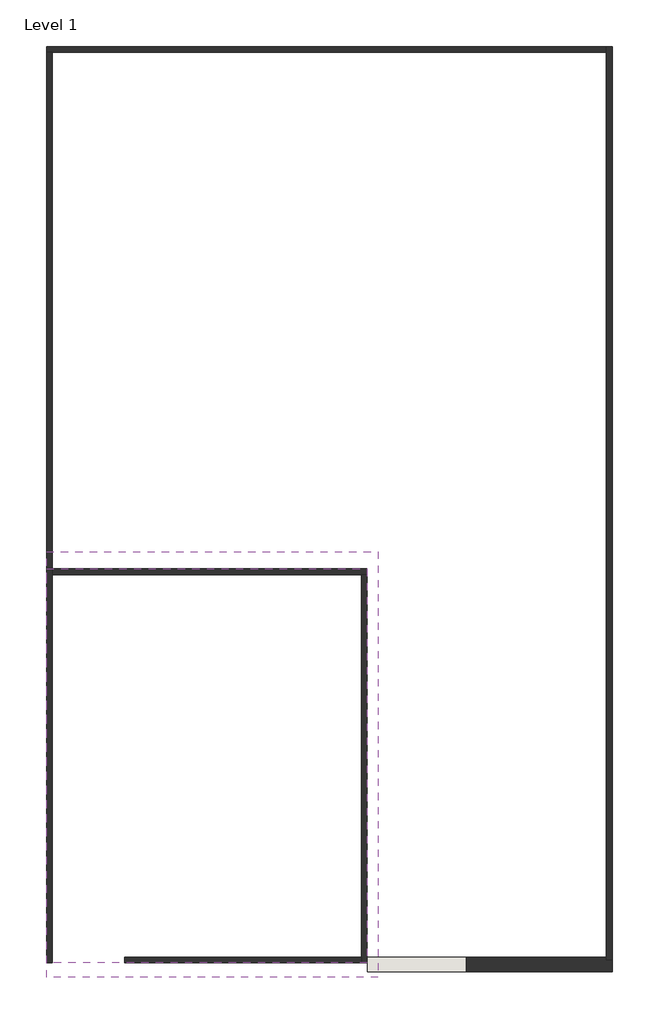
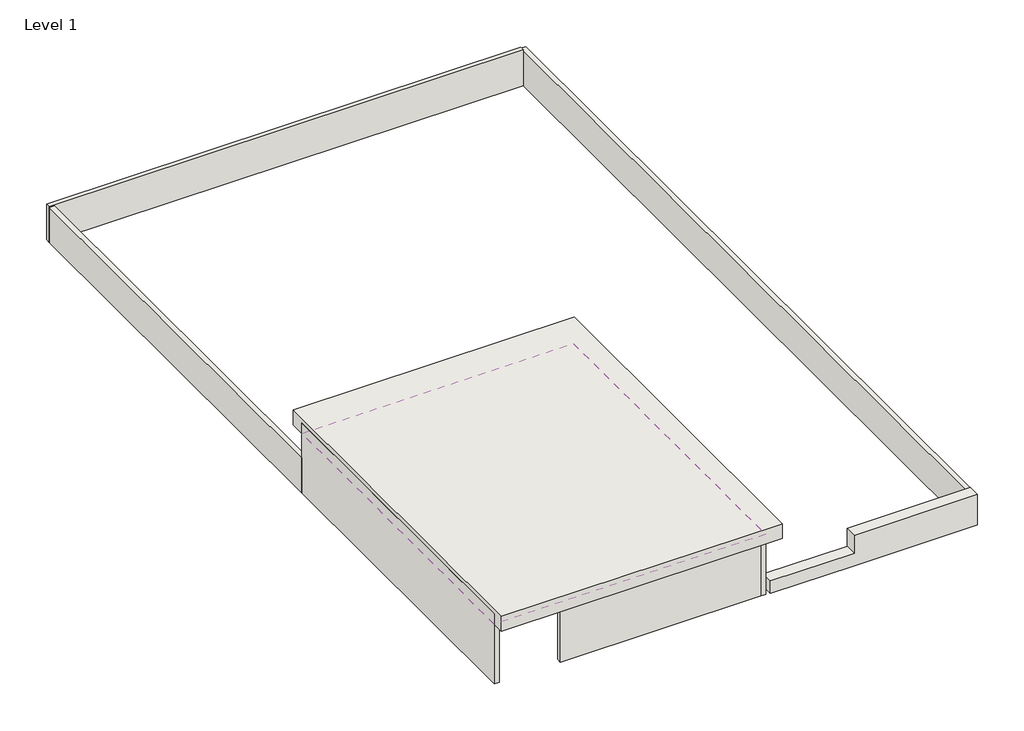
# One storey: 9 walls, 1 covering.
"""IFC4 building model written with IfcOpenShell, lengths in millimetres."""

from ifc_helpers import new_model, si_unit, frame, origin, place, context, project, spatial, polyline, outline, extrude, faceted_brep, transform, mapped, element, save
from components import walls_1_walls_1_3090deb3, walls_8_walls_8_6bca06a2

model = new_model("IFC4")

# Units and contexts
model_context = context("Model", 3, world=origin())
ifc_project = project(units=[si_unit("LENGTHUNIT", "METRE", prefix="MILLI")], contexts=[model_context])

# Site, building, storey
site = spatial("IfcSite", under=ifc_project)
building = spatial("IfcBuilding", under=site)
storey = spatial("IfcBuildingStorey", under=building, Name="Level 1", Elevation=3048.0)

# Covering
placement = place(None, origin())
element("IfcCovering", 1, ObjectType="600 x 1200mm grid", at=placement, inside=storey, context=model_context, shape_type="SweptSolid", body=[
    extrude(outline(polyline([(-7329.4383357, -6419.7210337), (-7329.4383357, -20130.9210337), (-18502.2383357, -20130.9210337), (-18502.2383357, -6419.7210337), (-7329.4383357, -6419.7210337)])), frame((0.0, 0.0, 5648.0), z_axis=(0.0, 0.0, 1.0), x_axis=(1.0, 0.0, 0.0)), (0.0, 0.0, 1.0), 52.0),
])

# Walls
element("IfcWall", 2, ObjectType="Generic - 9\"", at=placement, inside=storey, context=model_context, shape_type="SweptSolid", body=[
    extrude(outline(polyline([(-7529.4383357, -20130.9210337), (-15779.6883357, -20130.9210337), (-15779.6883357, -19930.9210337), (-7529.4383357, -19930.9210337), (-7529.4383357, -20130.9210337)])), frame((0.0, 0.0, 3048.0), z_axis=(0.0, 0.0, 1.0), x_axis=(1.0, 0.0, 0.0)), (0.0, 0.0, 1.0), 3048.0),
])
element("IfcWall", 3, ObjectType="Generic - 9\"", at=placement, inside=storey, context=model_context, shape_type="Brep", body=[
    faceted_brep([(-18502.2383357, -6419.7210337, 6096.0), (-18502.2383357, -6419.7210337, 4568.6541388), (-18502.2383357, -6419.7210337, 3048.0), (-18502.2383357, -20130.9210337, 3048.0), (-18502.2383357, -20130.9210337, 6096.0), (-18302.2383357, -6419.7210337, 3048.0), (-18302.2383357, -6419.7210337, 4568.6541388), (-18302.2383357, -6419.7210337, 6096.0), (-18302.2383357, -6619.7210337, 6096.0), (-18302.2383357, -20130.9210337, 6096.0), (-18302.2383357, -20130.9210337, 3048.0), (-18302.2383357, -6619.7210337, 3048.0)], [[[0, 1, 2, 3, 4]], [[5, 6, 7, 8, 9, 10, 11]], [[3, 2, 5, 11, 10]], [[4, 3, 10, 9]], [[0, 4, 9, 8, 7]], [[0, 7, 6, 5, 2, 1]]]),
])
element("IfcWall", 4, ObjectType="Generic - 9\"", at=placement, inside=storey, context=model_context, shape_type="Brep", body=[
    faceted_brep([(-7329.4383357, -6419.7210337, 3048.0), (-18302.2383357, -6419.7210337, 3048.0), (-18302.2383357, -6419.7210337, 6096.0), (-7329.4383357, -6419.7210337, 6096.0), (-7329.4383357, -6619.7210337, 3048.0), (-7329.4383357, -6619.7210337, 6096.0), (-7529.4383357, -6619.7210337, 6096.0), (-18302.2383357, -6619.7210337, 6096.0), (-18302.2383357, -6619.7210337, 3048.0), (-7529.4383357, -6619.7210337, 3048.0)], [[[0, 1, 2, 3]], [[4, 5, 6, 7, 8, 9]], [[1, 0, 4, 9, 8]], [[3, 2, 7, 6, 5]], [[0, 3, 5, 4]], [[1, 8, 7, 2]]]),
])
element("IfcWall", 5, ObjectType="Generic - 9\"", at=placement, inside=storey, context=model_context, shape_type="Brep", body=[
    faceted_brep([(-7329.4383357, -20130.9210337, 3048.0), (-7329.4383357, -6619.7210337, 3048.0), (-7329.4383357, -6619.7210337, 6096.0), (-7329.4383357, -20130.9210337, 6096.0), (-7529.4383357, -20130.9210337, 3048.0), (-7529.4383357, -20130.9210337, 6096.0), (-7529.4383357, -19930.9210337, 6096.0), (-7529.4383357, -6619.7210337, 6096.0), (-7529.4383357, -6619.7210337, 3048.0), (-7529.4383357, -19930.9210337, 3048.0)], [[[0, 1, 2, 3]], [[4, 5, 6, 7, 8, 9]], [[1, 0, 4, 9, 8]], [[3, 2, 7, 6, 5]], [[0, 3, 5, 4]], [[2, 1, 8, 7]]]),
])
element("IfcWall", 6, ObjectType="Generic - 9\"", at=placement, inside=storey, context=model_context, shape_type="Brep", body=[
    faceted_brep([(1204.9616643, -20030.9210337, 3048.0), (1204.9616643, 11768.2789663, 3048.0), (1204.9616643, 11768.2789663, 4552.0261891), (1204.9616643, -20030.9210337, 4552.0261891), (1004.9616643, -20030.9210337, 3048.0), (1004.9616643, -20030.9210337, 4552.0261891), (1004.9616643, 11768.2789663, 4552.0261891), (1004.9616643, 11768.2789663, 3048.0), (1004.9616643, 11568.2789663, 3048.0)], [[[0, 1, 2, 3]], [[4, 5, 6, 7, 8]], [[1, 0, 4, 8, 7]], [[3, 2, 6, 5]], [[0, 3, 5, 4]], [[2, 1, 7, 6]]]),
])
element("IfcWall", 7, ObjectType="Generic - 9\"", at=placement, inside=storey, context=model_context, shape_type="Brep", body=[
    faceted_brep([(1004.9616643, 11768.2789663, 3048.0), (-18502.2383357, 11768.2789663, 3048.0), (-18502.2383357, 11768.2789663, 4593.6791808), (1004.9616643, 11768.2789663, 4593.6791808), (1004.9616643, 11768.2789663, 4552.0261891), (1004.9616643, 11568.2789663, 3048.0), (1004.9616643, 11568.2789663, 4593.6791808), (-18502.2383357, 11568.2789663, 4593.6791808), (-18502.2383357, 11568.2789663, 4568.6541388), (-18502.2383357, 11568.2789663, 3048.0), (-18302.2383357, 11568.2789663, 3048.0)], [[[0, 1, 2, 3, 4]], [[5, 6, 7, 8, 9, 10]], [[1, 0, 5, 10, 9]], [[3, 2, 7, 6]], [[0, 4, 3, 6, 5]], [[2, 1, 9, 8, 7]]]),
])
element("IfcWall", 8, ObjectType="Generic - 9\"", at=placement, inside=storey, context=model_context, shape_type="SweptSolid", body=[
    extrude(outline(polyline([(-18302.2383357, 11568.2789663), (-18302.2383357, -6419.7210337), (-18502.2383357, -6419.7210337), (-18502.2383357, 11568.2789663), (-18302.2383357, 11568.2789663)])), frame((0.0, 0.0, 3048.0), z_axis=(0.0, 0.0, 1.0), x_axis=(1.0, 0.0, 0.0)), (0.0, 0.0, 1.0), 1520.6541388),
])
walls_1_walls_1_shape = walls_1_walls_1_3090deb3(model_context)
element("IfcWall", 9, ObjectType="Walls 1 : Walls 1", at=placement, inside=storey, context=model_context, shape_type="MappedRepresentation", body=[
    mapped(walls_1_walls_1_shape, transform((-2.5309138, -416.0770943, 0.0), x_axis=(1.0, 0.0, 0.0), y_axis=(0.0, 1.0, 0.0), z_axis=(0.0, 0.0, 1.0))),
])
walls_8_walls_8_shape = walls_8_walls_8_6bca06a2(model_context)
element("IfcWall", 10, ObjectType="Walls 8 : Walls 8", at=placement, inside=storey, context=model_context, shape_type="MappedRepresentation", body=[
    mapped(walls_8_walls_8_shape, transform((0.0, 0.0, 0.0), x_axis=(1.0, 0.0, 0.0), y_axis=(0.0, 1.0, 0.0), z_axis=(0.0, 0.0, 1.0))),
])

save(model, "model.ifc")

# Revit data of these elements
# Type "600 x 1200mm grid"
#   built-in parameter 1002203 = 1 (stored number, unit not read)
#   built-in parameter 1002202 = 1 (stored number, unit not read)
#   Layers, outside or top first: 0' - 1.41732" "Default" (function 1); 0' - 0.62992" "Ceiling Tile 600 x 1200" (function 5)
# Type "Generic - 9\""
#   Layers, outside or top first: 0' - 7.87402" no material (function 1)
# Element 1 (IfcCovering, "600 x 1200mm grid")
#   Height Offset From Level = 8' - 6.3622"
#   Phase Created = New Construction
#   Materials on its faces: "Ceiling Tile 600 x 1200", "Default"
# Elements 2, 3, 4, 5 (IfcWall, "Generic - 9\"")
#   Top Offset = 0' - 0"
#   Base Offset = 0' - 0"
#   Unconnected Height = 10' - 0"
#   wall height = 10' - 0"
#   Phase Created = New Construction
#   Base Constraint = Level 1
#   Materials on its faces: "Default Wall"
# Element 6 (IfcWall, "Generic - 9\"")
#   Top Offset = 0' - 0"
#   Base Offset = 0' - 0"
#   Unconnected Height = 4' - 11.21363"
#   wall height = 4' - 11.21363"
#   Phase Created = New Construction
#   Base Constraint = Level 1
#   Materials on its faces: "Default Wall"
# Element 7 (IfcWall, "Generic - 9\"")
#   Top Offset = 0' - 0"
#   Base Offset = 0' - 0"
#   Unconnected Height = 5' - 0.85351"
#   wall height = 5' - 0.85351"
#   Phase Created = New Construction
#   Base Constraint = Level 1
#   Materials on its faces: "Default Wall"
# Element 8 (IfcWall, "Generic - 9\"")
#   Top Offset = 0' - 0"
#   Base Offset = 0' - 0"
#   Unconnected Height = 4' - 11.86827"
#   wall height = 4' - 11.86827"
#   Phase Created = New Construction
#   Base Constraint = Level 1
#   Materials on its faces: "Default Wall"
# Element 9 (IfcWall, "Walls 1 : Walls 1")
#   Phase Created = New Construction
#   Materials on its faces: "Default Wall"
# Element 10 (IfcWall, "Walls 8 : Walls 8")
#   Phase Created = New Construction
#   Materials on its faces: "Default Wall"
# Materials
#   "Default": colour RGB 80 80 80, transparency 0
#   "Ceiling Tile 600 x 1200": class "Generic", colour RGB 179 178 175, transparency 0, Description = "Acoustic ceiling tile", Cost = 0
#   "Default Wall": colour RGB 80 80 80, transparency 0
